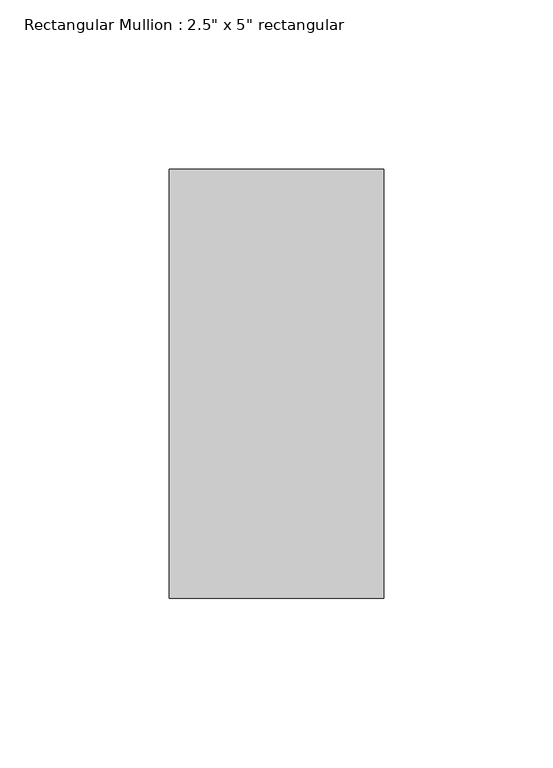
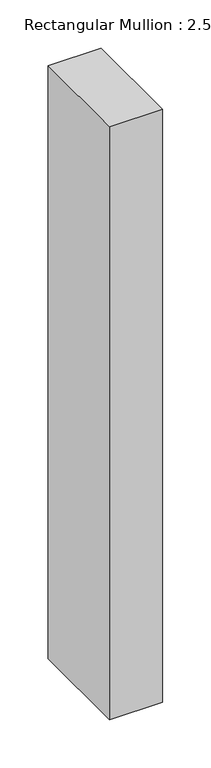
"""IFC4 building model written with IfcOpenShell, lengths in millimetres: member geometry."""

from ifc_helpers import new_model, si_unit, frame, origin, place, context, project, spatial, polyline, outline, extrude, source, transform, mapped, element, save


def member_5ade0aff(model_context):
    return source(origin(), model_context, "Body", "SweptSolid", [
        extrude(outline(polyline([(0.0, 63.5), (0.0, -63.5), (-63.5, -63.5), (-63.5, 63.5), (0.0, 63.5)])), frame((0.0, 0.0, -749.3168761), z_axis=(0.0, 0.0, 1.0), x_axis=(1.0, 0.0, 0.0)), (0.0, 0.0, 1.0), 749.3168761),
    ])


if __name__ == "__main__":
    model = new_model("IFC4")
    model_context = context("Model", 3, world=origin())
    ifc_project = project(units=[si_unit("LENGTHUNIT", "METRE", prefix="MILLI")], contexts=[model_context])
    site = spatial("IfcSite", under=ifc_project)
    building = spatial("IfcBuilding", under=site)
    placement = place(None, origin())
    member_shape = member_5ade0aff(model_context)
    element("IfcMember", 1, ObjectType="Rectangular Mullion : 2.5\" x 5\" rectangular", at=placement, inside=building, context=model_context, shape_type="MappedRepresentation", body=[
        mapped(member_shape, transform((0.0, 0.0, 0.0), x_axis=(1.0, 0.0, 0.0), y_axis=(0.0, 1.0, 0.0), z_axis=(0.0, 0.0, 1.0))),
    ])
    save(model, "model.ifc")

# Revit data of these elements
# Type "Rectangular Mullion : 2.5\" x 5\" rectangular"
#   built-in parameter 1007304 = 0.416667 (stored number, unit not read)
#   built-in parameter 1007301 = 0.104167 (stored number, unit not read)
#   built-in parameter 1007300 = 0.104167 (stored number, unit not read)
# Element 1 (IfcMember, "Rectangular Mullion : 2.5\" x 5\" rectangular")
#   Materials on its faces: "Aluminum"
# Materials
#   "Aluminum": class "Metal", colour RGB 247 247 247, transparency 0, Description = "Aluminum 6061", Cost = 0
